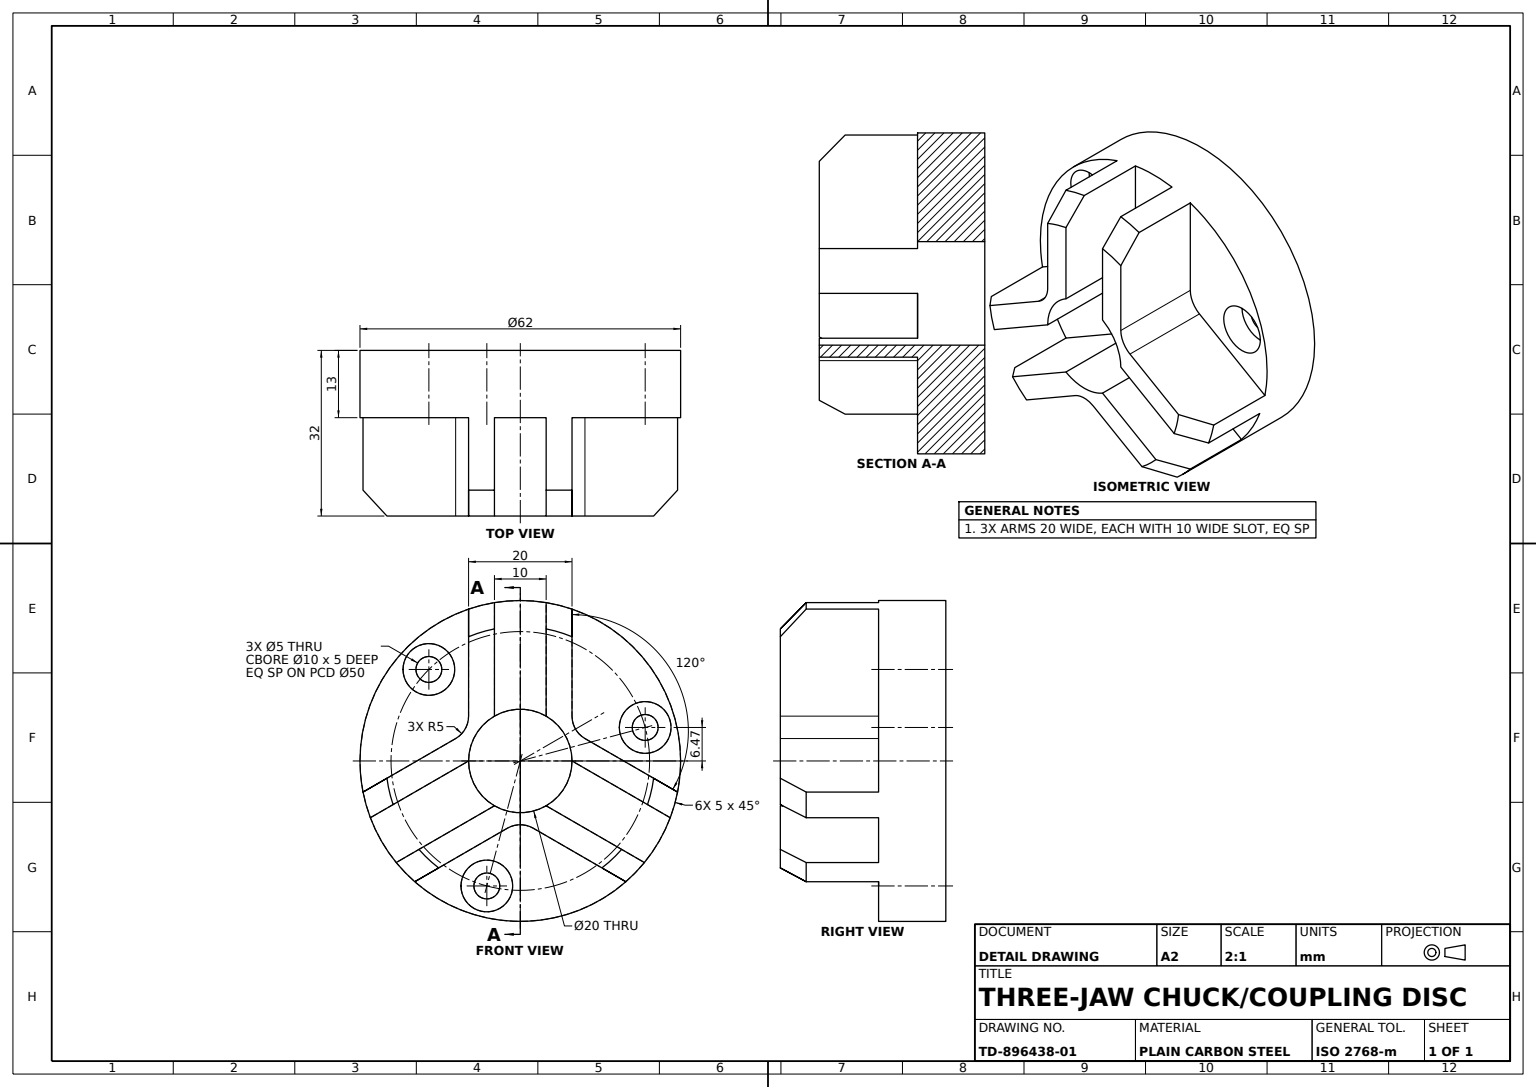
from build123d import *

# Parameters (mm, degrees)
BASE_DISC_SKETCH_R        = 31
BASE_DISC_62_DEPTH        = 13
RELIEF_CUT_SKETCH_R       = 10
RELIEF_CUT_DEPTH          = 46.727453461
THREE_ARM_BOSS_DEPTH      = 19
ARM_GAP_SKETCH_R          = 2.5
ARM_GAP_CUT_DEPTH         = 48.780749262
RADIAL_HOLE_SKETCH_R      = 5
RADIAL_HOLE_10_DEPTH      = 5
ARM_CUTS_PATTERN_3X_COUNT = 3
ARM_CHAMFERS_5MM_SIZE     = 5


with BuildPart() as part:
    # Base Disc Sketch → Base Disc Ø62 (new body)
    with BuildSketch(Plane.XY):
        with Locations(Location((0, 0, 0), (0, 0, 180))):
            Circle(BASE_DISC_SKETCH_R)
    extrude(amount=BASE_DISC_62_DEPTH)

    # Relief Cut Sketch → Relief Cut (cut, through all)
    with BuildSketch(Plane.XY.offset(13)):
        Circle(RELIEF_CUT_SKETCH_R)
    extrude(amount=-RELIEF_CUT_DEPTH, mode=Mode.SUBTRACT)

    # Arms Profile Sketch → Three-Arm Boss (add)
    with BuildSketch(Plane.XY.offset(13)):
        with BuildLine():
            Line((-5, 8.660254038), (-5, 30.594117082))
            ThreePointArc((-5, 30.594117082), (-7.526051267, 30.072554802), (-10, 29.342801502))
            Line((-10, 29.342801502), (-10, 8.660254038))
            ThreePointArc((-10, 8.660254038), (-10.669872981, 6.160254038), (-12.5, 4.330127019))
            Line((-12.5, 4.330127019), (-30.411611519, -6.011146713))
            ThreePointArc((-30.411611519, -6.011146713), (-29.806622049, -8.518525814), (-28.995282599, -10.966931522))
            Line((-28.995282599, -10.966931522), (-10, 0))
            ThreePointArc((-10, 0), (-8.660254038, 5), (-5, 8.660254038))
        make_face()
        with BuildLine():
            ThreePointArc((12.5, 4.330127019), (10.669872981, 6.160254038), (10, 8.660254038))
            Line((10, 8.660254038), (10, 29.342801502))
            ThreePointArc((10, 29.342801502), (7.526051267, 30.072554802), (5, 30.594117082))
            Line((5, 30.594117082), (5, 8.660254038))
            ThreePointArc((5, 8.660254038), (8.660254038, 5), (10, 0))
            Line((10, 0), (28.995282599, -10.966931522))
            ThreePointArc((28.995282599, -10.966931522), (29.806622049, -8.518525814), (30.411611519, -6.011146713))
            Line((30.411611519, -6.011146713), (12.5, 4.330127019))
        make_face()
        with BuildLine():
            ThreePointArc((20.411611519, -23.331654789), (22.280570782, -21.554028988), (23.995282599, -19.62718556))
            Line((23.995282599, -19.62718556), (5, -8.660254038))
            ThreePointArc((5, -8.660254038), (0, -10), (-5, -8.660254038))
            Line((-5, -8.660254038), (-23.995282599, -19.62718556))
            ThreePointArc((-23.995282599, -19.62718556), (-22.280570782, -21.554028988), (-20.411611519, -23.331654789))
            Line((-20.411611519, -23.331654789), (-2.5, -12.990381057))
            ThreePointArc((-2.5, -12.990381057), (0, -12.320508076), (2.5, -12.990381057))
            Line((2.5, -12.990381057), (20.411611519, -23.331654789))
        make_face()
    extrude(amount=THREE_ARM_BOSS_DEPTH)

    # Arm Gap Sketch → Arm Gap Cut (cut, through all)
    with BuildSketch(Plane.XY.offset(13)):
        with Locations((-6.470476128, -24.148145657)):
            Circle(ARM_GAP_SKETCH_R)
    arm_gap_cut = extrude(amount=-ARM_GAP_CUT_DEPTH, mode=Mode.SUBTRACT)

    # Radial Hole Sketch → Radial Hole Ø10 (cut)
    with BuildSketch(Plane.XY.offset(13)):
        with Locations((-6.470476128, -24.148145657)):
            Circle(RADIAL_HOLE_SKETCH_R)
    radial_hole_10 = extrude(amount=-RADIAL_HOLE_10_DEPTH, mode=Mode.SUBTRACT)

    # Arm Cuts Pattern 3x: Arm Gap Cut, Radial Hole Ø10 ×3 about axis
    arm_cuts_pattern_3x_axis = Axis((0, 0, 0), (0, 0, 1))
    add([arm_gap_cut.rotate(arm_cuts_pattern_3x_axis, i * 360 / ARM_CUTS_PATTERN_3X_COUNT) for i in range(1, ARM_CUTS_PATTERN_3X_COUNT)], mode=Mode.SUBTRACT)
    add([radial_hole_10.rotate(arm_cuts_pattern_3x_axis, i * 360 / ARM_CUTS_PATTERN_3X_COUNT) for i in range(1, ARM_CUTS_PATTERN_3X_COUNT)], mode=Mode.SUBTRACT)

    # Arm Chamfers 5mm
    arm_chamfers_5mm_edges = [part.edges().sort_by_distance(p)[0] for p in [
        (-29.806622049, -8.518525814, 32),
        (-7.526051267, 30.072554802, 32),
        (7.526051267, 30.072554802, 32),
        (29.806622049, -8.518525814, 32),
        (22.280570782, -21.554028988, 32),
        (-22.280570782, -21.554028988, 32),
    ]]
    chamfer(arm_chamfers_5mm_edges, length=ARM_CHAMFERS_5MM_SIZE)


solid = part.part
